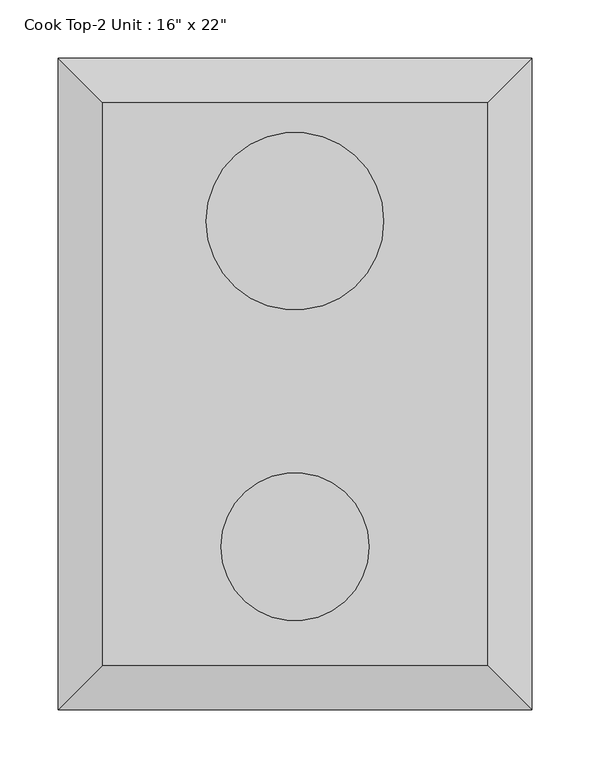
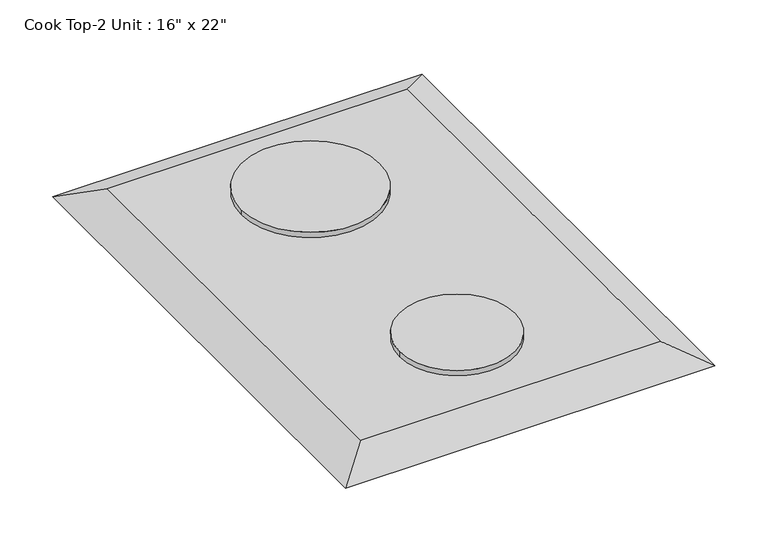
"""IFC4 building model written with IfcOpenShell, lengths in millimetres: proxy geometry."""

from ifc_helpers import new_model, si_unit, point, frame, frame_2d, origin, place, context, project, spatial, circle_curve, trimmed, segment, composite_curve, outline, extrude, faceted_brep, source, transform, mapped, element, save


def proxy_caef4acf(model_context):
    return source(origin(), model_context, "Body", "SolidModel", [
        faceted_brep([(241.3, 271.5247956, 806.45), (-88.9, 271.5247956, 806.45), (-88.9, -211.0752044, 806.45), (241.3, -211.0752044, 806.45), (279.4, 309.6247956, 787.4), (279.4, -249.1752044, 787.4), (-127.0, -249.1752044, 787.4), (-127.0, 309.6247956, 787.4)], [[[0, 1, 2, 3]], [[4, 5, 6, 7]], [[4, 7, 1, 0]], [[7, 6, 2, 1]], [[6, 5, 3, 2]], [[5, 4, 0, 3]]]),
        extrude(outline(composite_curve([segment(trimmed(circle_curve(frame_2d((76.2, 169.9247956)), 76.2), [point((152.4, 169.9247956))], [point((0.0, 169.9247956))], False, "CARTESIAN"), True, "CONTINUOUS"), segment(trimmed(circle_curve(frame_2d((76.2, 169.9247956)), 76.2), [point((0.0, 169.9247956))], [point((152.4, 169.9247956))], False, "CARTESIAN"), True, "CONTINUOUS")], self_intersect=False)), frame((0.0, 0.0, 806.45), z_axis=(0.0, 0.0, 1.0), x_axis=(1.0, 0.0, 0.0)), (0.0, 0.0, 1.0), 6.35),
        extrude(outline(composite_curve([segment(trimmed(circle_curve(frame_2d((76.2, -109.4752044)), 63.5), [point((139.7, -109.4752044))], [point((12.7, -109.4752044))], False, "CARTESIAN"), True, "CONTINUOUS"), segment(trimmed(circle_curve(frame_2d((76.2, -109.4752044)), 63.5), [point((12.7, -109.4752044))], [point((139.7, -109.4752044))], False, "CARTESIAN"), True, "CONTINUOUS")], self_intersect=False)), frame((0.0, 0.0, 806.45), z_axis=(0.0, 0.0, 1.0), x_axis=(1.0, 0.0, 0.0)), (0.0, 0.0, 1.0), 6.35),
    ])


if __name__ == "__main__":
    model = new_model("IFC4")
    model_context = context("Model", 3, world=origin())
    ifc_project = project(units=[si_unit("LENGTHUNIT", "METRE", prefix="MILLI")], contexts=[model_context])
    site = spatial("IfcSite", under=ifc_project)
    building = spatial("IfcBuilding", under=site)
    placement = place(None, origin())
    proxy_shape = proxy_caef4acf(model_context)
    element("IfcBuildingElementProxy", 1, Name="Cook Top-2 Unit : 16\" x 22\"", ObjectType="Cook Top-2 Unit : 16\" x 22\"", at=placement, inside=building, context=model_context, shape_type="MappedRepresentation", body=[
        mapped(proxy_shape, transform((0.0, 0.0, 0.0), x_axis=(1.0, 0.0, 0.0), y_axis=(0.0, 1.0, 0.0), z_axis=(0.0, 0.0, 1.0))),
    ])
    save(model, "model.ifc")

# Revit data of these elements
# Type "Cook Top-2 Unit : 16\" x 22\""
#   Assembly Code = "E1090400"
#   Counter Height = 2.583333 ft
#   Depth = 1.833333 ft
#   Width = 1.333333 ft
#   Burner Material = Metal - Chrome
#   Cooktop Material = Metal - Steel, Polished
#   Default Elevation = 0
# Element 1 (IfcBuildingElementProxy, "Cook Top-2 Unit : 16\" x 22\"")
#   Materials on its faces: "Metal - Steel, Polished", "Metal - Chrome"
# Materials
#   "Metal - Chrome": class "Metal", colour RGB 247 247 247, transparency 0
#   "Metal - Steel, Polished": colour RGB 57 57 57, transparency 0
